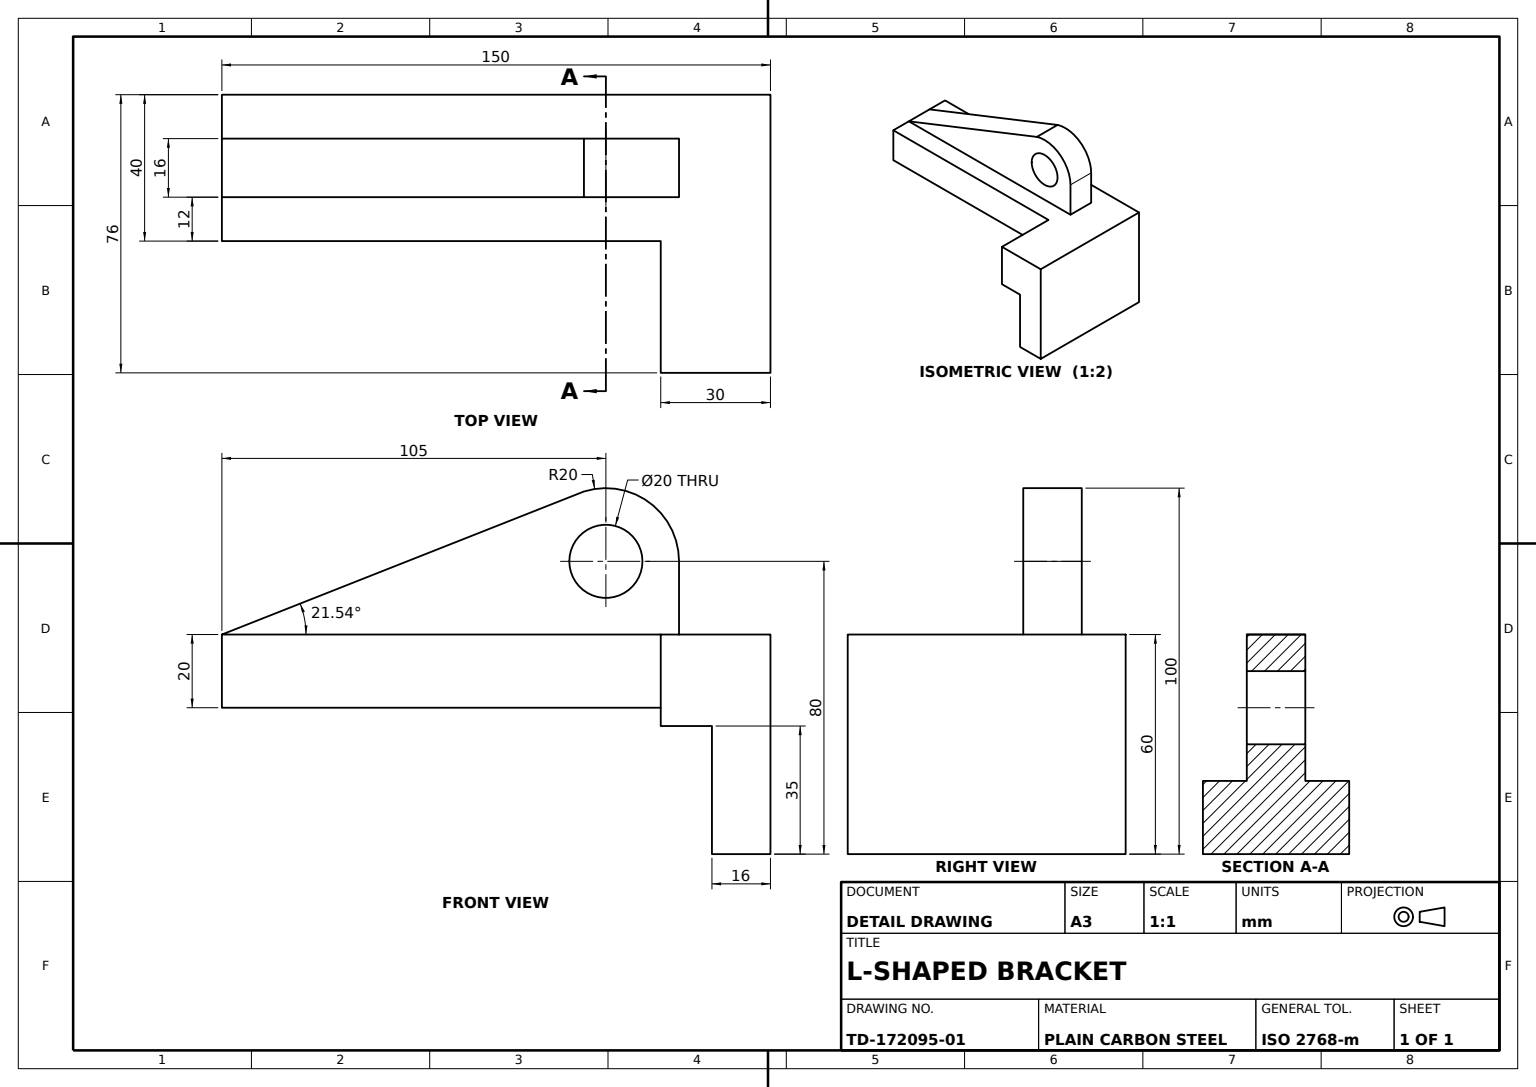
SolidWorks part; units mm, degrees
material "Plain Carbon Steel"
ref_plane "Front Plane" through (0, 0, 0) normal (0, 0, 1) x (1, 0, 0)
ref_plane "Top Plane" through (0, 0, 0) normal (0, 1, 0) x (1, 0, 0)
ref_plane "Right Plane" through (0, 0, 0) normal (1, 0, 0) x (0, 0, -1)
sketch "Base Plate Sketch" plane through (0, 0, 0) normal (0, 0, 1) x (1, 0, 0)
  line L0 (0, 0) -> (76, 0)
  line L1 (76, 0) -> (76, 60)
  line L2 (76, 60) -> (0, 60)
  line L3 (0, 60) -> (0, 0)
  dimension "D1" = 76
  dimension "D2" = 60
extrude "Base Plate" add sketch "Base Plate Sketch" along normal blind 16
sketch "Upright Wall Sketch" plane through (76, 0, 0) normal (1, 0, 0) x (0, 0, -1)
  line L0 (-16, 60) -> (-41, 60)
  line L1 (-41, 60) -> (-46, 60)
  line L2 (-46, 60) -> (-46, 35)
  line L3 (-46, 35) -> (-16, 35)
  line L4 (-16, 0) -> (-16, 60) construction
  line L5 (-16, 35) -> (-16, 60)
  line L6 (0, 0) -> (0, 60) construction
  dimension "D1" = 41
  dimension "D2" = 46
extrude "Upright Wall" add sketch "Upright Wall Sketch" against normal blind 76
sketch "Wall Notch Sketch" plane through (0, 0, 46) normal (0, 0, 1) x (1, 0, 0)
  line L0 (0, 60) -> (76, 60)
  line L1 (76, 60) -> (76, 35)
  line L2 (76, 35) -> (0, 35)
  line L3 (0, 35) -> (0, 60)
extrude "Wall Notch" cut sketch "Wall Notch Sketch" against normal blind 16
sketch "Arm Block Sketch" plane through (0, 0, 0) normal (-1, 0, 0) x (0, 0, 1)
  line L0 (30, 60) -> (150, 60)
  line L1 (150, 60) -> (150, 40)
  line L2 (150, 40) -> (30, 40)
  line L3 (30, 60) -> (30, 35) construction
  line L4 (30, 40) -> (30, 60)
  line L5 (30, 35) -> (16, 35) construction
  dimension "D1" = 120
  dimension "D2" = 5
extrude "Arm Block" add sketch "Arm Block Sketch" against normal blind 40
sketch "Arm Lug Sketch" plane through (40, 0, 0) normal (1, 0, 0) x (0, 0, -1)
  line L0 (-150, 60) -> (-25, 60)
  line L1 (-30, 60) -> (-30, 40) construction
  line L3 (-25, 80) -> (-25, 60)
  line L4 (-150, 60) -> (-50.9995, 99.0789)
  arc A0 (-25, 80) -> (-53.6498, 98.0328) centre (-45, 80) ccw
  line M3 (-30, 60) -> (-150, 60)
  dimension "D1" = 20
  dimension "D2" = 40
  dimension "D3" = 5
  dimension "D4" = 20.9995
extrude "Arm Lug" add sketch "Arm Lug Sketch" against normal blind 40 contours L3 A0 L4 L0 M3
sketch "Arm Side Cut A Sketch" plane through (40, 0, 0) normal (1, 0, 0) x (0, 0, -1)
  line L0 (-150, 60) -> (-25, 60)
  line L1 (-25, 60) -> (-25, 80)
  line L2 (-150, 60) -> (-50.9995, 99.0789)
  arc A0 (-25, 80) -> (-53.6498, 98.0328) centre (-45, 80) ccw
  line M2 (-30, 60) -> (-25, 60)
  line M3 (-25, 60) -> (-25, 80)
  arc M4 (-25, 80) -> (-50.9995, 99.0789) centre (-45, 80) ccw
  line M5 (-50.9995, 99.0789) -> (-150, 60)
  dimension "D1" = 40
extrude "Arm Side Cut A" cut sketch "Arm Side Cut A Sketch" against normal blind 12 contours L2 L0 M5 M2 M3 M4
sketch "Arm Side Cut B Sketch" plane through (0, 0, 0) normal (-1, 0, 0) x (0, 0, 1)
  line L0 (25, 60) -> (150, 60)
  line L1 (150, 60) -> (50.9995, 99.0789)
  line L2 (25, 60) -> (25, 80)
  line L3 (25, 80) -> (25, 60) construction
  arc A0 (50.9995, 99.0789) -> (25, 80) centre (45, 80) ccw construction
  arc A1 (53.6498, 98.0328) -> (25, 80) centre (45, 80) ccw
  line M5 (150, 60) -> (50.9995, 99.0789)
  arc M6 (50.9995, 99.0789) -> (25, 80) centre (45, 80) ccw
  line M7 (25, 80) -> (25, 60)
  dimension "D1" = 40
extrude "Arm Side Cut B" cut sketch "Arm Side Cut B Sketch" against normal blind 12 contours L0 L1 M7 M5 M6
sketch "Pivot Hole Ø20 Sketch" plane through (28, 0, 0) normal (1, 0, 0) x (0, 0, -1)
  circle A0 centre (-45, 80) radius 10
  dimension "D1" = 20
  dimension "D2" = 20
extrude "Pivot Hole Ø20" cut sketch "Pivot Hole Ø20 Sketch" against normal blind 16
